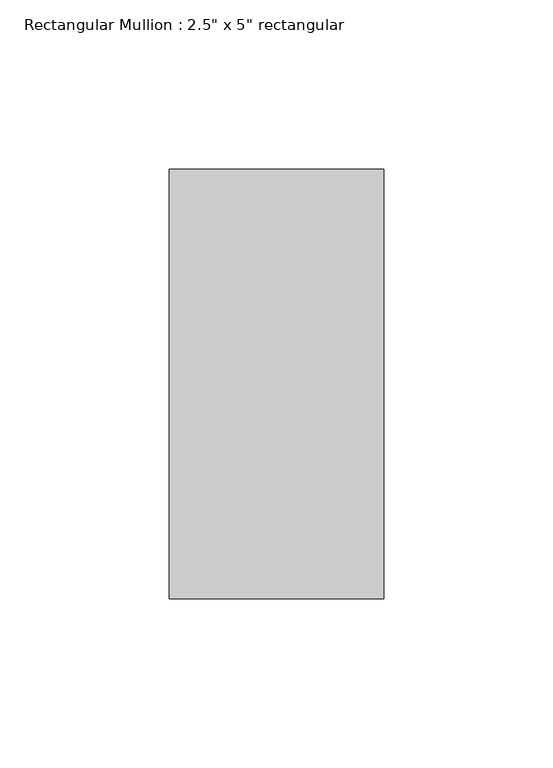
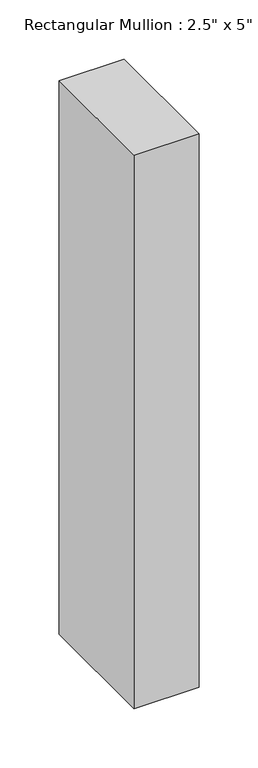
"""IFC4 building model written with IfcOpenShell, lengths in millimetres: member geometry."""

from ifc_helpers import new_model, si_unit, frame, origin, place, context, project, spatial, polyline, outline, extrude, source, transform, mapped, element, save


def member_de12db52(model_context):
    return source(origin(), model_context, "Body", "SweptSolid", [
        extrude(outline(polyline([(31.75, 63.5), (31.75, -63.5), (-31.75, -63.5), (-31.75, 63.5), (31.75, 63.5)])), frame((0.0, 0.0, -571.5), z_axis=(0.0, 0.0, 1.0), x_axis=(1.0, 0.0, 0.0)), (0.0, 0.0, 1.0), 571.5),
    ])


if __name__ == "__main__":
    model = new_model("IFC4")
    model_context = context("Model", 3, world=origin())
    ifc_project = project(units=[si_unit("LENGTHUNIT", "METRE", prefix="MILLI")], contexts=[model_context])
    site = spatial("IfcSite", under=ifc_project)
    building = spatial("IfcBuilding", under=site)
    placement = place(None, origin())
    member_shape = member_de12db52(model_context)
    element("IfcMember", 1, ObjectType="Rectangular Mullion : 2.5\" x 5\" rectangular", at=placement, inside=building, context=model_context, shape_type="MappedRepresentation", body=[
        mapped(member_shape, transform((0.0, 0.0, 0.0), x_axis=(1.0, 0.0, 0.0), y_axis=(0.0, 1.0, 0.0), z_axis=(0.0, 0.0, 1.0))),
    ])
    save(model, "model.ifc")

# Revit data of these elements
# Type "Rectangular Mullion : 2.5\" x 5\" rectangular"
#   built-in parameter 1007304 = 0.416667 (stored number, unit not read)
#   built-in parameter 1007301 = 0.104167 (stored number, unit not read)
#   built-in parameter 1007300 = 0.104167 (stored number, unit not read)
# Element 1 (IfcMember, "Rectangular Mullion : 2.5\" x 5\" rectangular")
#   Materials on its faces: "Aluminum"
# Materials
#   "Aluminum": class "Metal", colour RGB 247 247 247, transparency 0, Description = "Aluminum 6061", Cost = 0
